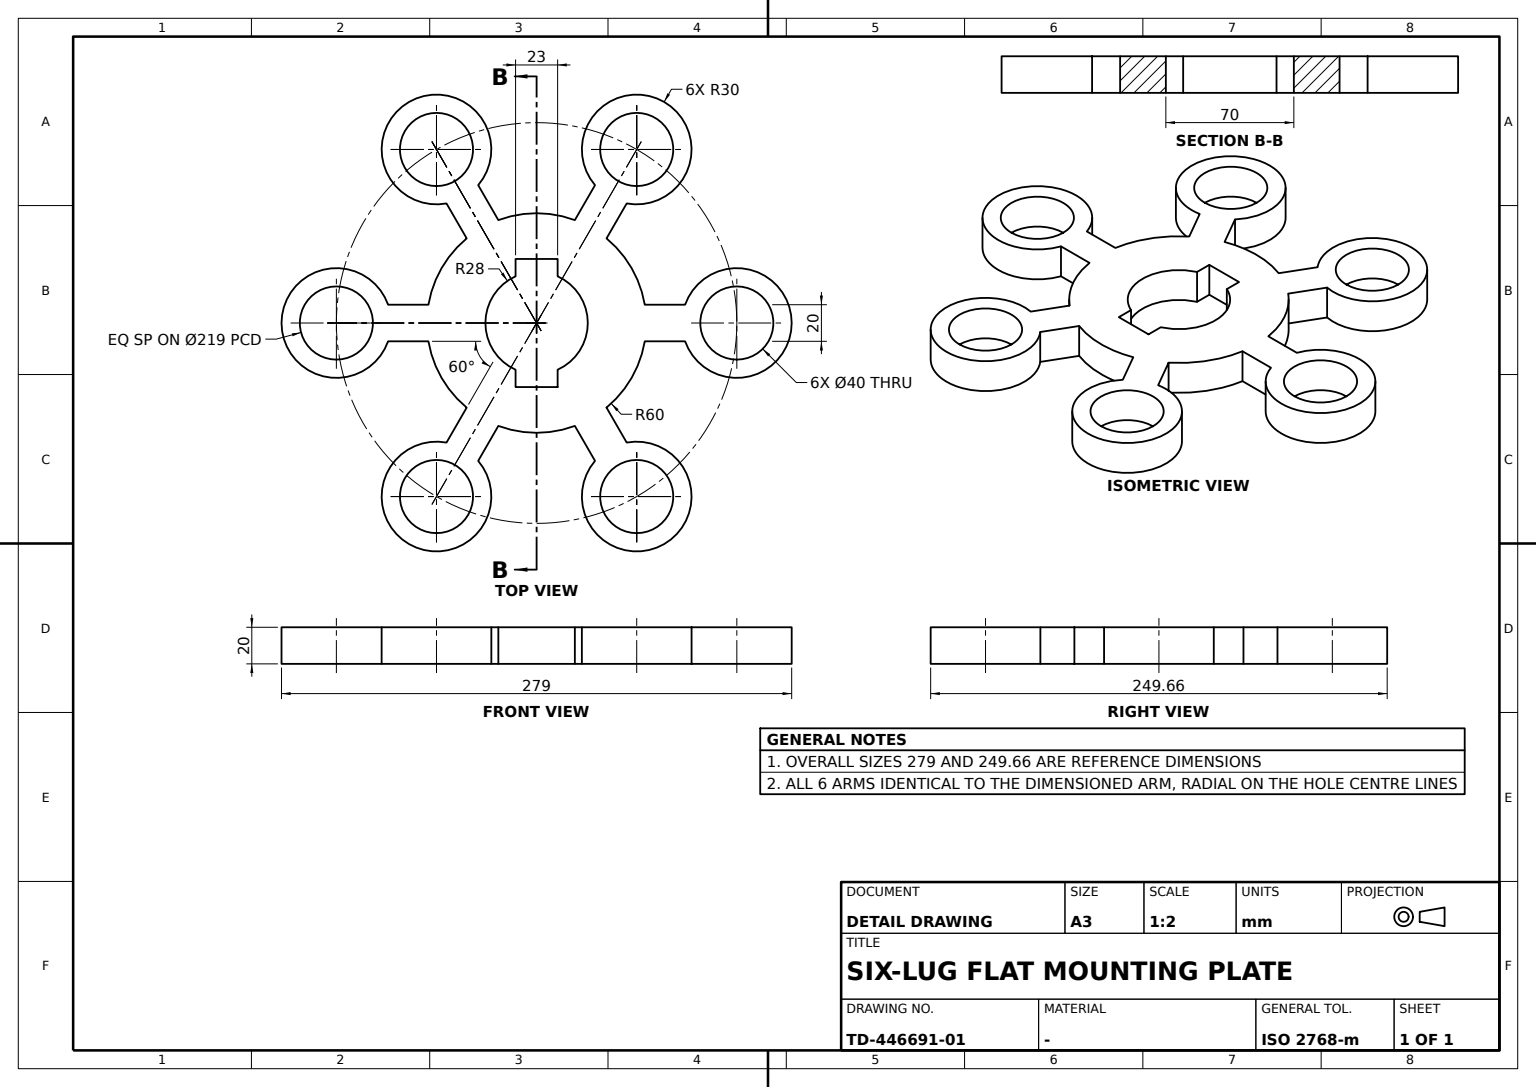
CATIA V5 part; units mm, degrees
sketch "Sketch1" plane through (0, 0, 0) normal (0, 0, 1) x (1, 0, 0)
  arc A0 (46.2348, 38.2407) -> (10, 59.1608) centre (0, 0) ccw
  line L0 (35, 11.5) -> (35, -11.5)
  line L1 (35, -11.5) -> (25.5294, -11.5)
  line L2 (-35, -11.5) -> (-35, 11.5)
  line L3 (-35, 11.5) -> (-25.5294, 11.5)
  arc A1 (25.5294, 11.5) -> (-25.5294, 11.5) centre (0, 0) ccw
  line L4 (25.5294, 11.5) -> (35, 11.5)
  line L5 (-25.5294, -11.5) -> (-35, -11.5)
  point P0 (-25.5294, -11.5)
  arc A2 (-25.5294, -11.5) -> (25.5294, -11.5) centre (0, 0) ccw
  circle A3 centre (0, 0) radius 109.5 construction
  line L6 (0, 0) -> (158.4419, 91.4765) construction
  arc A4 (75.3349, 31.9476) -> (65.3349, 49.2681) centre (94.8298, 54.75) ccw
  point P1 (94.8298, 54.75)
  line L7 (45.3712, 26.1951) -> (80.042, 46.2123) construction
  point P2 (45.3712, 26.1951)
  point P3 (80.042, 46.2123)
  line L8 (56.2348, 20.9201) -> (75.3349, 31.9476)
  line L9 (45.3712, 26.1951) -> (50.3712, 17.5348) construction
  line L10 (80.042, 46.2123) -> (85.042, 37.552) construction
  line L11 (46.2348, 38.2407) -> (65.3349, 49.2681)
  line L12 (45.3712, 26.1951) -> (40.3712, 34.8554) construction
  line L13 (80.042, 46.2123) -> (75.042, 54.8726) construction
  circle A5 centre (94.8298, 54.75) radius 20
  circle A6 centre (0, 109.5) radius 20
  point P4 (0, 109.5)
  arc A7 (10, 81.2157) -> (-10, 81.2157) centre (0, 109.5) ccw
  line L14 (0, 49.2681) -> (0, 79.5) construction
  point P5 (0, 49.2681)
  point P6 (0, 89.5)
  line L15 (-10, 59.1608) -> (-10, 81.2157)
  line L16 (0, 49.2681) -> (-10, 49.2681) construction
  line L17 (0, 89.5) -> (-10, 89.5) construction
  line L18 (10, 59.1608) -> (10, 81.2157)
  line L19 (0, 49.2681) -> (10, 49.2681) construction
  line L20 (0, 89.5) -> (10, 89.5) construction
  point P7 (-10, 59.1608)
  arc A8 (-10, 59.1608) -> (-46.2348, 38.2407) centre (0, 0) ccw
  circle A9 centre (-94.8298, 54.75) radius 20
  point P8 (-94.8298, 54.75)
  arc A10 (-65.3349, 49.2681) -> (-75.3349, 31.9476) centre (-94.8298, 54.75) ccw
  line L21 (0, 0) -> (-94.8298, 54.75) construction
  line L22 (-44.683, 25.7978) -> (-77.5093, 44.75) construction
  point P9 (-44.683, 25.7978)
  point P10 (-77.5093, 44.75)
  line L23 (-56.2348, 20.9201) -> (-75.3349, 31.9476)
  line L24 (-44.683, 25.7978) -> (-49.683, 17.1375) construction
  line L25 (-77.5093, 44.75) -> (-82.5093, 36.0897) construction
  line L26 (-46.2348, 38.2407) -> (-65.3349, 49.2681)
  point P11 (-39.683, 34.458)
  line L27 (-44.683, 25.7978) -> (-39.683, 34.458) construction
  line L28 (-77.5093, 44.75) -> (-72.5093, 53.4103) construction
  point P12 (-56.2348, 20.9201)
  arc A11 (-56.2348, 20.9201) -> (-56.2348, -20.9201) centre (0, 0) ccw
  arc A12 (-75.3349, -31.9476) -> (-65.3349, -49.2681) centre (-94.8298, -54.75) ccw
  point P13 (-94.8298, -54.75)
  circle A13 centre (-94.8298, -54.75) radius 20
  point P14 (-83.2898, -71.0849)
  line L29 (0, 0) -> (-94.8298, -54.75) construction
  line L30 (-77.5093, -44.75) -> (-45.9127, -26.5077) construction
  point P15 (-77.5093, -44.75)
  line L31 (-65.3349, -49.2681) -> (-46.2348, -38.2407)
  line L32 (-77.5093, -44.75) -> (-72.5093, -53.4103) construction
  line L33 (-45.9127, -26.5077) -> (-40.9127, -35.168) construction
  line L34 (-75.3349, -31.9476) -> (-56.2348, -20.9201)
  line L35 (-77.5093, -44.75) -> (-82.5093, -36.0897) construction
  line L36 (-45.9127, -26.5077) -> (-50.9127, -17.8475) construction
  point P16 (-46.2348, -38.2407)
  arc A14 (-46.2348, -38.2407) -> (-10, -59.1608) centre (0, 0) ccw
  circle A15 centre (0, -109.5) radius 20
  point P17 (0, -109.5)
  arc A16 (-10, -81.2157) -> (10, -81.2157) centre (0, -109.5) ccw
  line L37 (0, -89.5) -> (0, -51.0393) construction
  point P18 (0, -89.5)
  line L38 (10, -81.2157) -> (10, -59.1608)
  line L39 (0, -89.5) -> (10, -89.5) construction
  line L40 (0, -51.0393) -> (10, -51.0393) construction
  line L41 (-10, -81.2157) -> (-10, -59.1608)
  line L42 (0, -89.5) -> (-10, -89.5) construction
  line L43 (0, -51.0393) -> (-10, -51.0393) construction
  point P19 (10, -59.1608)
  arc A17 (10, -59.1608) -> (46.2348, -38.2407) centre (0, 0) ccw
  circle A18 centre (94.8298, -54.75) radius 20
  point P20 (94.8298, -54.75)
  arc A19 (65.3349, -49.2681) -> (75.3349, -31.9476) centre (94.8298, -54.75) ccw
  point P21 (114.3247, -77.5524)
  line L44 (77.5093, -44.75) -> (45.3712, -26.1951) construction
  point P22 (77.5093, -44.75)
  line L45 (75.3349, -31.9476) -> (56.2348, -20.9201)
  line L46 (77.5093, -44.75) -> (82.5093, -36.0897) construction
  line L47 (45.3712, -26.1951) -> (50.3712, -17.5348) construction
  line L48 (65.3349, -49.2681) -> (46.2348, -38.2407)
  point P23 (56.2348, -20.9201)
  arc A20 (56.2348, -20.9201) -> (56.2348, 20.9201) centre (0, 0) ccw
  dimension "radius A0" = 60
  dimension "distance y axis L2" = 35
  dimension "length L0" = 23
  dimension "radius A1" = 28
  dimension "radius A3" = 109.5
  dimension "angle L6 x axis" = 30
  dimension "radius A4" = 30
  dimension "distance L7 L8" = 10
  dimension "distance L7 L11" = 10
  dimension "radius A5" = 20
  dimension "radius A6" = 20
  dimension "radius A7" = 30
  dimension "distance L14 L15" = 10
  dimension "distance L14 L18" = 10
  dimension "radius A9" = 20
  dimension "radius A10" = 30
  dimension "angle L21 x axis" = 30
  dimension "distance L22 L23" = 10
  dimension "distance L22 L26" = 10
  dimension "radius A13" = 20
  dimension "radius A12" = 30
  dimension "angle L29 y axis" = 120
  dimension "distance L30 L31" = 10
  dimension "distance L30 L34" = 10
  dimension "radius A15" = 20
  dimension "radius A16" = 30
  dimension "distance L37 L38" = 10
  dimension "distance L37 L41" = 10
  dimension "radius A18" = 20
  dimension "radius A19" = 30
  dimension "distance L44 L45" = 10
  dimension "length L48" = 22.0549
  constraint vertical L0 y-axis
  constraint vertical L2 y-axis
  constraint vertical L14 y-axis
  constraint vertical L37 y-axis
  constraint horizontal L1 x-axis
  constraint horizontal L3 x-axis
  constraint horizontal L4 x-axis
  constraint horizontal L5 x-axis
  constraint equidistance L0 L2 origin
  constraint equidistance L1 L3 origin
  constraint coincidence L3 L4
  constraint coincidence A1 P0
  constraint coincidence L1 L5
  constraint coincidence A1 A2
  constraint coincidence P1 L6
  constraint coincidence P1 A3
  constraint coincidence P2 L6
  constraint coincidence P3 L6
  constraint coincidence P4 A3
  constraint coincidence P4 y-axis
  constraint coincidence P5 y-axis
  constraint coincidence P6 A6
  constraint coincidence A0 P7
  constraint coincidence A0 A8
  constraint coincidence P8 A3
  constraint coincidence P9 L21
  constraint coincidence P10 A9
  constraint coincidence A8 P12
  constraint coincidence A8 A11
  constraint coincidence P13 A3
  constraint coincidence A13 P14
  constraint coincidence P14 A3
  constraint coincidence P15 A13
  constraint coincidence P15 L29
  constraint coincidence A11 P16
  constraint coincidence A11 A14
  constraint coincidence P17 A3
  constraint coincidence P17 y-axis
  constraint coincidence P18 A15
  constraint coincidence P18 y-axis
  constraint coincidence A14 P19
  constraint coincidence A14 A17
  constraint coincidence P20 L21
  constraint coincidence P20 A3
  constraint coincidence A19 P21
  constraint coincidence P21 L23
  constraint coincidence P22 A18
  constraint coincidence P22 L22
  constraint coincidence L45 P11
  constraint coincidence L48 P21
  constraint coincidence A17 P23
  constraint coincidence A17 A20
  constraint perpendicularity L9 L7
  constraint perpendicularity L9 L8
  constraint perpendicularity L10 L7
  constraint perpendicularity L10 L8
  constraint perpendicularity L12 L7
  constraint perpendicularity L12 L11
  constraint perpendicularity L13 L7
  constraint perpendicularity L13 L11
  constraint perpendicularity L16 L14
  constraint perpendicularity L16 L15
  constraint perpendicularity L17 L14
  constraint perpendicularity L17 L15
  constraint perpendicularity L19 L14
  constraint perpendicularity L19 L18
  constraint perpendicularity L20 L14
  constraint perpendicularity L20 L18
  constraint perpendicularity L24 L22
  constraint perpendicularity L24 L23
  constraint perpendicularity L25 L22
  constraint perpendicularity L25 L23
  constraint perpendicularity L27 L22
  constraint perpendicularity L27 L26
  constraint perpendicularity L28 L22
  constraint perpendicularity L28 L26
  constraint perpendicularity L32 L30
  constraint perpendicularity L32 L31
  constraint perpendicularity L33 L30
  constraint perpendicularity L33 L31
  constraint perpendicularity L35 L30
  constraint perpendicularity L35 L34
  constraint perpendicularity L36 L30
  constraint perpendicularity L36 L34
  constraint perpendicularity L39 L37
  constraint perpendicularity L39 L38
  constraint perpendicularity L40 L37
  constraint perpendicularity L40 L38
  constraint perpendicularity L42 L37
  constraint perpendicularity L42 L41
  constraint perpendicularity L43 L37
  constraint perpendicularity L43 L41
  constraint perpendicularity L46 L44
  constraint perpendicularity L46 L45
  constraint perpendicularity L47 L44
  constraint perpendicularity L47 L45
  constraint parallelism L22 L21
  constraint parallelism L30 L6
  constraint parallelism L44 L22
extrude "Pad1" add sketch "Sketch1" along normal mid plane 20
